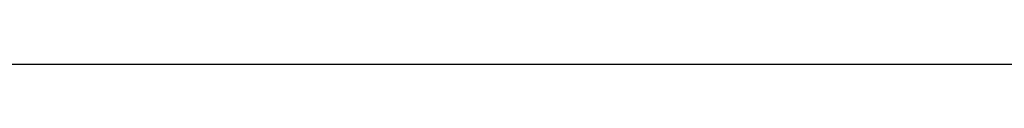
# Model space of a CAD drawing. Units: inches. Extents: x 459864 to 460310, y 324185 to 324787.
# Tile 100 of 112: x 460248.739 to 460250.864, y 324283.483 to 324283.483. Entities that reach past the tile are written whole.
import ezdxf

# ---------------------------------------------------------------- set-up
doc = ezdxf.new("R2010")
doc.units = ezdxf.units.IN
for name, color, linetype, lineweight in [('A-ANNO-DIMS', 2, 'Continuous', 18), ('L-HRDS', 9, 'Continuous', 18), ('L-SITE-PATT', 252, 'Continuous', 13)]:
    doc.layers.add(name, color=color, linetype=linetype, lineweight=lineweight)
doc.styles.get("Standard").update_dxf_attribs({"font": 'arial.ttf'})
doc.dimstyles.new('ISO-25', dxfattribs={"dimtxt": 6, "dimasz": 2.5, "dimexe": 1.25, "dimexo": 0.625, "dimtad": 1, "dimdec": 1, "dimlunit": 3, "dimtxsty": 'Standard', "dimcen": 2.5, "dimadec": 0, "dimazin": 0, "dimtfac": 1, "dimtdec": 1, "dimtmove": 0, "dimatfit": 3, "dimfxl": 1, "dimarcsym": 0})

# ---------------------------------------------------------------- blocks, each defined once
blk = doc.blocks.new('*D21')
at = {"layer": 'A-ANNO-DIMS', "color": 0, "lineweight": -2, "transparency": 16777216}
for p, q in [((460247.7399, 324715.4832), (460309.5804, 324715.4832)), ((460308.3304, 324712.9832), (460308.3304, 324285.9832)), ((460247.7399, 324283.4832), (460309.5804, 324283.4832))]:
    blk.add_line(p, q, dxfattribs=at)
at = {"layer": 'A-ANNO-DIMS', "color": 0, "transparency": 16777216}
for points in [[(460307.9137, 324712.9832), (460308.747, 324712.9832), (460308.3304, 324715.4832)], [(460307.9137, 324285.9832), (460308.747, 324285.9832), (460308.3304, 324283.4832)]]:
    blk.add_solid(points, dxfattribs=at)
at = {"layer": 'Defpoints', "color": 0, "transparency": 16777216}
for p in [(460247.1149, 324715.4832), (460247.1149, 324283.4832), (460308.3304, 324283.4832)]:
    blk.add_point(p, dxfattribs=at)
at = {"layer": 'A-ANNO-DIMS', "color": 0, "transparency": 16777216, "insert": (460304.6399, 324499.4832), "char_height": 6, "attachment_point": 5, "rotation": 90}
blk.add_mtext("36'", dxfattribs=at)

msp = doc.modelspace()

# ---------------------------------------------------------------- hatches: boundary and pattern name
at = {"layer": 'L-SITE-PATT'}
h = msp.add_hatch(dxfattribs=at)
h.set_pattern_fill('DOTS', color=256)
h.paths.add_polyline_path([(460269.8036, 324283.4832), (460247.1149, 324283.4832), (460121.9293, 324283.4832), (460121.9293, 324252.473), (460117.4293, 324252.473), (460110.1236, 324252.473), (460110.1236, 324243.2865), (460080.8295, 324243.2865), (460080.8295, 324252.473), (460061.1149, 324252.473), (460061.1149, 324251.8824), (460077.9089, 324251.8824), (460077.9089, 324199.4832), (460080.8295, 324199.4832), (460080.8295, 324207.5532), (460110.1236, 324207.5532), (460110.1236, 324199.4832), (460110.8133, 324199.4832), (460262.1149, 324199.4832), (460269.8036, 324199.4832)], flags=17)
edge = h.paths.add_edge_path(flags=0)
edge.add_ellipse((460222.5903, 324263.8132), major_axis=(-8.4853, 8.4853), ratio=1, start_angle=405, end_angle=495, ccw=False)
edge.add_line((460214.8209, 324254.6599), (460214.8316, 324254.6659))
edge.add_ellipse((460222.5903, 324263.8132), major_axis=(-8.4853, 8.4853), ratio=1, start_angle=405, end_angle=495, ccw=False)
edge.add_line((460210.7589, 324261.7806), (460210.7676, 324261.7868))
edge.add_ellipse((460222.5903, 324263.8132), major_axis=(-8.4853, 8.4853), ratio=1, start_angle=405, end_angle=495, ccw=False)
edge.add_ellipse((460222.5903, 324263.8132), major_axis=(-8.4853, 8.4853), ratio=1, start_angle=392.75402, end_angle=405, ccw=False)
edge.add_ellipse((460222.5903, 324263.8132), major_axis=(-8.4853, 8.4853), ratio=1, start_angle=380.93472, end_angle=392.75402, ccw=False)
edge.add_line((460211.3371, 324267.985), (460211.3404, 324267.985))
edge.add_ellipse((460222.5903, 324263.8132), major_axis=(-8.4853, 8.4853), ratio=1, start_angle=380.93472, end_angle=392.75402, ccw=False)
edge.add_ellipse((460222.5903, 324263.8132), major_axis=(-8.4853, 8.4853), ratio=1, start_angle=347.90152, end_angle=380.93472, ccw=False)
edge.add_ellipse((460222.5903, 324263.8132), major_axis=(-8.4853, 8.4853), ratio=1, start_angle=327.06192, end_angle=347.90152, ccw=False)
edge.add_ellipse((460222.5903, 324263.8132), major_axis=(-8.4853, 8.4853), ratio=1, start_angle=278.32464, end_angle=327.06192, ccw=False)
edge.add_line((460225.1583, 324275.536), (460225.1577, 324275.5346))
edge.add_ellipse((460222.5903, 324263.8132), major_axis=(-8.4853, 8.4853), ratio=1, start_angle=278.32464, end_angle=327.06192, ccw=False)
edge.add_ellipse((460222.5903, 324263.8132), major_axis=(-8.4853, 8.4853), ratio=1, start_angle=260.64357, end_angle=278.32464, ccw=False)
edge.add_ellipse((460222.5903, 324263.8132), major_axis=(-8.4853, 8.4853), ratio=1, start_angle=225, end_angle=260.64357, ccw=False)
edge.add_line((460234.5088, 324265.2428), (460234.5015, 324265.2394))
edge.add_ellipse((460222.5903, 324263.8132), major_axis=(-8.4853, 8.4853), ratio=1, start_angle=225, end_angle=260.64357, ccw=False)
edge.add_ellipse((460222.5903, 324263.8132), major_axis=(-8.4853, 8.4853), ratio=1, start_angle=495, end_angle=585, ccw=False)
edge.add_line((460234.4367, 324261.8612), (460234.4238, 324261.8578))
edge.add_ellipse((460222.5903, 324263.8132), major_axis=(-8.4853, 8.4853), ratio=1, start_angle=495, end_angle=585, ccw=False)
edge.add_line((460227.9501, 324253.0672), (460227.9464, 324253.0831))
edge.add_ellipse((460222.5903, 324263.8132), major_axis=(-8.4853, 8.4853), ratio=1, start_angle=495, end_angle=585, ccw=False)
edge.add_line((460226.223, 324252.3693), (460226.211, 324252.3796))
edge.add_ellipse((460222.5903, 324263.8132), major_axis=(-8.4853, 8.4853), ratio=1, start_angle=495, end_angle=585, ccw=False)
h.paths.add_polyline_path([(460219.6515, 324254.3467), (460218.4613, 324253.545), (460218.2754, 324254.7893), (460219.6424, 324256.5418), (460219.6246, 324260.8476), (460216.1101, 324257.333), (460214.35, 324256.9781), (460215.4164, 324259.3557), (460212.5239, 324258.4958), (460213.1373, 324259.9298), (460218.5072, 324263.8132), (460222.5903, 324263.8132), (460222.5903, 324267.8067), (460218.1755, 324272.2123), (460219.026, 324274.639), (460222.5903, 324272.8111), (460222.5903, 324275.4233), (460223.0571, 324274.8249), (460222.6752, 324273.4922), (460225.9117, 324267.1346), (460219.6246, 324260.8476)], flags=0)
edge = h.paths.add_edge_path(flags=0)
edge.add_ellipse((460194.5758, 324264.0465), major_axis=(-8.4853, 8.4853), ratio=1, start_angle=495, end_angle=585, ccw=False)
edge.add_line((460199.9356, 324253.3005), (460199.9319, 324253.3164))
edge.add_ellipse((460194.5758, 324264.0465), major_axis=(-8.4853, 8.4853), ratio=1, start_angle=495, end_angle=585, ccw=False)
edge.add_line((460198.2084, 324252.6025), (460198.1965, 324252.6128))
edge.add_ellipse((460194.5758, 324264.0465), major_axis=(-8.4853, 8.4853), ratio=1, start_angle=495, end_angle=585, ccw=False)
edge.add_ellipse((460194.5758, 324264.0465), major_axis=(-8.4853, 8.4853), ratio=1, start_angle=405, end_angle=495, ccw=False)
edge.add_line((460186.8063, 324254.8932), (460186.8171, 324254.8992))
edge.add_ellipse((460194.5758, 324264.0465), major_axis=(-8.4853, 8.4853), ratio=1, start_angle=405, end_angle=495, ccw=False)
edge.add_line((460182.7444, 324262.0138), (460182.753, 324262.0201))
edge.add_ellipse((460194.5758, 324264.0465), major_axis=(-8.4853, 8.4853), ratio=1, start_angle=405, end_angle=495, ccw=False)
edge.add_ellipse((460194.5758, 324264.0465), major_axis=(-8.4853, 8.4853), ratio=1, start_angle=392.75402, end_angle=405, ccw=False)
edge.add_ellipse((460194.5758, 324264.0465), major_axis=(-8.4853, 8.4853), ratio=1, start_angle=380.93472, end_angle=392.75402, ccw=False)
edge.add_line((460183.3225, 324268.2183), (460183.3259, 324268.2183))
edge.add_ellipse((460194.5758, 324264.0465), major_axis=(-8.4853, 8.4853), ratio=1, start_angle=380.93472, end_angle=392.75402, ccw=False)
edge.add_ellipse((460194.5758, 324264.0465), major_axis=(-8.4853, 8.4853), ratio=1, start_angle=347.90152, end_angle=380.93472, ccw=False)
edge.add_ellipse((460194.5758, 324264.0465), major_axis=(-8.4853, 8.4853), ratio=1, start_angle=327.06192, end_angle=347.90152, ccw=False)
edge.add_ellipse((460194.5758, 324264.0465), major_axis=(-8.4853, 8.4853), ratio=1, start_angle=278.32464, end_angle=327.06192, ccw=False)
edge.add_line((460197.1437, 324275.7693), (460197.1432, 324275.7679))
edge.add_ellipse((460194.5758, 324264.0465), major_axis=(-8.4853, 8.4853), ratio=1, start_angle=278.32464, end_angle=327.06192, ccw=False)
edge.add_ellipse((460194.5758, 324264.0465), major_axis=(-8.4853, 8.4853), ratio=1, start_angle=260.64357, end_angle=278.32464, ccw=False)
edge.add_ellipse((460194.5758, 324264.0465), major_axis=(-8.4853, 8.4853), ratio=1, start_angle=225, end_angle=260.64357, ccw=False)
edge.add_line((460206.4943, 324265.4761), (460206.4869, 324265.4727))
edge.add_ellipse((460194.5758, 324264.0465), major_axis=(-8.4853, 8.4853), ratio=1, start_angle=225, end_angle=260.64357, ccw=False)
edge.add_ellipse((460194.5758, 324264.0465), major_axis=(-8.4853, 8.4853), ratio=1, start_angle=495, end_angle=585, ccw=False)
edge.add_line((460206.4221, 324262.0945), (460206.4092, 324262.0911))
h.paths.add_polyline_path([(460191.6101, 324261.0808), (460191.6369, 324254.5799), (460190.4468, 324253.7783), (460190.2609, 324255.0226), (460191.6279, 324256.775), (460191.6101, 324261.0808), (460188.0956, 324257.5663), (460186.3354, 324257.2113), (460187.4018, 324259.5889), (460184.5094, 324258.7291), (460185.1228, 324260.1631), (460190.4927, 324264.0465), (460194.5758, 324264.0465), (460194.5758, 324268.04), (460190.161, 324272.4456), (460191.0114, 324274.8722), (460194.5758, 324273.0444), (460194.5758, 324275.6566), (460195.0426, 324275.0582), (460194.6607, 324273.7255), (460197.8971, 324267.3679)], flags=0)
edge = h.paths.add_edge_path(flags=0)
edge.add_ellipse((460252.912, 324263.5776), major_axis=(-8.4853, 8.4853), ratio=1, start_angle=405, end_angle=495, ccw=False)
edge.add_line((460241.0806, 324261.5449), (460241.0892, 324261.5512))
edge.add_ellipse((460252.912, 324263.5776), major_axis=(-8.4853, 8.4853), ratio=1, start_angle=405, end_angle=495, ccw=False)
edge.add_ellipse((460252.912, 324263.5776), major_axis=(-8.4853, 8.4853), ratio=1, start_angle=392.75402, end_angle=405, ccw=False)
edge.add_ellipse((460252.912, 324263.5776), major_axis=(-8.4853, 8.4853), ratio=1, start_angle=380.93472, end_angle=392.75402, ccw=False)
edge.add_line((460241.6587, 324267.7494), (460241.6621, 324267.7494))
edge.add_ellipse((460252.912, 324263.5776), major_axis=(-8.4853, 8.4853), ratio=1, start_angle=380.93472, end_angle=392.75402, ccw=False)
edge.add_ellipse((460252.912, 324263.5776), major_axis=(-8.4853, 8.4853), ratio=1, start_angle=347.90152, end_angle=380.93472, ccw=False)
edge.add_ellipse((460252.912, 324263.5776), major_axis=(-8.4853, 8.4853), ratio=1, start_angle=327.06192, end_angle=347.90152, ccw=False)
edge.add_ellipse((460252.912, 324263.5776), major_axis=(-8.4853, 8.4853), ratio=1, start_angle=278.32464, end_angle=327.06192, ccw=False)
edge.add_line((460255.4799, 324275.3004), (460255.4794, 324275.299))
edge.add_ellipse((460252.912, 324263.5776), major_axis=(-8.4853, 8.4853), ratio=1, start_angle=278.32464, end_angle=327.06192, ccw=False)
edge.add_ellipse((460252.912, 324263.5776), major_axis=(-8.4853, 8.4853), ratio=1, start_angle=260.64357, end_angle=278.32464, ccw=False)
edge.add_ellipse((460252.912, 324263.5776), major_axis=(-8.4853, 8.4853), ratio=1, start_angle=225, end_angle=260.64357, ccw=False)
edge.add_line((460264.8305, 324265.0072), (460264.8231, 324265.0038))
edge.add_ellipse((460252.912, 324263.5776), major_axis=(-8.4853, 8.4853), ratio=1, start_angle=225, end_angle=260.64357, ccw=False)
edge.add_ellipse((460252.912, 324263.5776), major_axis=(-8.4853, 8.4853), ratio=1, start_angle=495, end_angle=585, ccw=False)
edge.add_line((460264.7583, 324261.6256), (460264.7454, 324261.6222))
edge.add_ellipse((460252.912, 324263.5776), major_axis=(-8.4853, 8.4853), ratio=1, start_angle=495, end_angle=585, ccw=False)
edge.add_line((460258.2718, 324252.8316), (460258.2681, 324252.8475))
edge.add_ellipse((460252.912, 324263.5776), major_axis=(-8.4853, 8.4853), ratio=1, start_angle=495, end_angle=585, ccw=False)
edge.add_line((460256.5446, 324252.1337), (460256.5327, 324252.1439))
edge.add_ellipse((460252.912, 324263.5776), major_axis=(-8.4853, 8.4853), ratio=1, start_angle=495, end_angle=585, ccw=False)
edge.add_ellipse((460252.912, 324263.5776), major_axis=(-8.4853, 8.4853), ratio=1, start_angle=405, end_angle=495, ccw=False)
edge.add_line((460245.1425, 324254.4243), (460245.1533, 324254.4303))
h.paths.add_polyline_path([(460244.6716, 324256.7425), (460245.738, 324259.1201), (460242.8456, 324258.2602), (460243.459, 324259.6942), (460248.8289, 324263.5776), (460252.912, 324263.5776), (460252.912, 324267.5711), (460248.4972, 324271.9767), (460249.3476, 324274.4034), (460252.912, 324272.5755), (460252.912, 324275.1877), (460253.3788, 324274.5893), (460252.9969, 324273.2566), (460256.2333, 324266.899), (460249.9463, 324260.612), (460249.9731, 324254.111), (460248.783, 324253.3094), (460248.5971, 324254.5537), (460249.9641, 324256.3062), (460249.9463, 324260.612), (460246.4318, 324257.0974)], flags=0)
edge = h.paths.add_edge_path(flags=0)
edge.add_ellipse((460167.4387, 324262.8328), major_axis=(-8.4853, 8.4853), ratio=1, start_angle=495, end_angle=585, ccw=False)
edge.add_line((460172.7985, 324252.0868), (460172.7948, 324252.1027))
edge.add_ellipse((460167.4387, 324262.8328), major_axis=(-8.4853, 8.4853), ratio=1, start_angle=495, end_angle=585, ccw=False)
edge.add_line((460171.0714, 324251.3888), (460171.0594, 324251.3991))
edge.add_ellipse((460167.4387, 324262.8328), major_axis=(-8.4853, 8.4853), ratio=1, start_angle=495, end_angle=585, ccw=False)
edge.add_ellipse((460167.4387, 324262.8328), major_axis=(-8.4853, 8.4853), ratio=1, start_angle=405, end_angle=495, ccw=False)
edge.add_line((460159.6693, 324253.6795), (460159.68, 324253.6855))
edge.add_ellipse((460167.4387, 324262.8328), major_axis=(-8.4853, 8.4853), ratio=1, start_angle=405, end_angle=495, ccw=False)
edge.add_line((460155.6073, 324260.8001), (460155.616, 324260.8064))
edge.add_ellipse((460167.4387, 324262.8328), major_axis=(-8.4853, 8.4853), ratio=1, start_angle=405, end_angle=495, ccw=False)
edge.add_ellipse((460167.4387, 324262.8328), major_axis=(-8.4853, 8.4853), ratio=1, start_angle=392.75402, end_angle=405, ccw=False)
edge.add_ellipse((460167.4387, 324262.8328), major_axis=(-8.4853, 8.4853), ratio=1, start_angle=380.93472, end_angle=392.75402, ccw=False)
edge.add_line((460156.1855, 324267.0046), (460156.1888, 324267.0046))
edge.add_ellipse((460167.4387, 324262.8328), major_axis=(-8.4853, 8.4853), ratio=1, start_angle=380.93472, end_angle=392.75402, ccw=False)
edge.add_ellipse((460167.4387, 324262.8328), major_axis=(-8.4853, 8.4853), ratio=1, start_angle=347.90152, end_angle=380.93472, ccw=False)
edge.add_ellipse((460167.4387, 324262.8328), major_axis=(-8.4853, 8.4853), ratio=1, start_angle=327.06192, end_angle=347.90152, ccw=False)
edge.add_ellipse((460167.4387, 324262.8328), major_axis=(-8.4853, 8.4853), ratio=1, start_angle=278.32464, end_angle=327.06192, ccw=False)
edge.add_line((460170.0067, 324274.5556), (460170.0061, 324274.5542))
edge.add_ellipse((460167.4387, 324262.8328), major_axis=(-8.4853, 8.4853), ratio=1, start_angle=278.32464, end_angle=327.06192, ccw=False)
edge.add_ellipse((460167.4387, 324262.8328), major_axis=(-8.4853, 8.4853), ratio=1, start_angle=260.64357, end_angle=278.32464, ccw=False)
edge.add_ellipse((460167.4387, 324262.8328), major_axis=(-8.4853, 8.4853), ratio=1, start_angle=225, end_angle=260.64357, ccw=False)
edge.add_line((460179.3572, 324264.2624), (460179.3499, 324264.259))
edge.add_ellipse((460167.4387, 324262.8328), major_axis=(-8.4853, 8.4853), ratio=1, start_angle=225, end_angle=260.64357, ccw=False)
edge.add_ellipse((460167.4387, 324262.8328), major_axis=(-8.4853, 8.4853), ratio=1, start_angle=495, end_angle=585, ccw=False)
edge.add_line((460179.2851, 324260.8808), (460179.2722, 324260.8774))
h.paths.add_polyline_path([(460164.473, 324259.8671), (460164.4998, 324253.3662), (460163.3097, 324252.5645), (460163.1238, 324253.8089), (460164.4908, 324255.5613), (460164.473, 324259.8671), (460160.9585, 324256.3526), (460159.1984, 324255.9976), (460160.2648, 324258.3752), (460157.3723, 324257.5154), (460157.9857, 324258.9494), (460163.3556, 324262.8328), (460167.4387, 324262.8328), (460167.4387, 324266.8263), (460163.0239, 324271.2319), (460163.8744, 324273.6585), (460167.4387, 324271.8307), (460167.4387, 324274.4429), (460167.9055, 324273.8445), (460167.5236, 324272.5118), (460170.7601, 324266.1542)], flags=0)
edge = h.paths.add_edge_path(flags=0)
edge.add_ellipse((460140.7581, 324262.3696), major_axis=(-8.4853, 8.4853), ratio=1, start_angle=495, end_angle=585, ccw=False)
edge.add_line((460146.1179, 324251.6235), (460146.1142, 324251.6395))
edge.add_ellipse((460140.7581, 324262.3696), major_axis=(-8.4853, 8.4853), ratio=1, start_angle=495, end_angle=585, ccw=False)
edge.add_line((460144.3908, 324250.9256), (460144.3788, 324250.9359))
edge.add_ellipse((460140.7581, 324262.3696), major_axis=(-8.4853, 8.4853), ratio=1, start_angle=495, end_angle=585, ccw=False)
edge.add_ellipse((460140.7581, 324262.3696), major_axis=(-8.4853, 8.4853), ratio=1, start_angle=405, end_angle=495, ccw=False)
edge.add_line((460132.9887, 324253.2162), (460132.9994, 324253.2223))
edge.add_ellipse((460140.7581, 324262.3696), major_axis=(-8.4853, 8.4853), ratio=1, start_angle=405, end_angle=495, ccw=False)
edge.add_line((460128.9267, 324260.3369), (460128.9354, 324260.3432))
edge.add_ellipse((460140.7581, 324262.3696), major_axis=(-8.4853, 8.4853), ratio=1, start_angle=405, end_angle=495, ccw=False)
edge.add_ellipse((460140.7581, 324262.3696), major_axis=(-8.4853, 8.4853), ratio=1, start_angle=392.75402, end_angle=405, ccw=False)
edge.add_ellipse((460140.7581, 324262.3696), major_axis=(-8.4853, 8.4853), ratio=1, start_angle=380.93472, end_angle=392.75402, ccw=False)
edge.add_line((460129.5049, 324266.5414), (460129.5082, 324266.5414))
edge.add_ellipse((460140.7581, 324262.3696), major_axis=(-8.4853, 8.4853), ratio=1, start_angle=380.93472, end_angle=392.75402, ccw=False)
edge.add_ellipse((460140.7581, 324262.3696), major_axis=(-8.4853, 8.4853), ratio=1, start_angle=347.90152, end_angle=380.93472, ccw=False)
edge.add_ellipse((460140.7581, 324262.3696), major_axis=(-8.4853, 8.4853), ratio=1, start_angle=327.06192, end_angle=347.90152, ccw=False)
edge.add_ellipse((460140.7581, 324262.3696), major_axis=(-8.4853, 8.4853), ratio=1, start_angle=278.32464, end_angle=327.06192, ccw=False)
edge.add_line((460143.3261, 324274.0923), (460143.3255, 324274.091))
edge.add_ellipse((460140.7581, 324262.3696), major_axis=(-8.4853, 8.4853), ratio=1, start_angle=278.32464, end_angle=327.06192, ccw=False)
edge.add_ellipse((460140.7581, 324262.3696), major_axis=(-8.4853, 8.4853), ratio=1, start_angle=260.64357, end_angle=278.32464, ccw=False)
edge.add_ellipse((460140.7581, 324262.3696), major_axis=(-8.4853, 8.4853), ratio=1, start_angle=225, end_angle=260.64357, ccw=False)
edge.add_line((460152.6766, 324263.7992), (460152.6692, 324263.7958))
edge.add_ellipse((460140.7581, 324262.3696), major_axis=(-8.4853, 8.4853), ratio=1, start_angle=225, end_angle=260.64357, ccw=False)
edge.add_ellipse((460140.7581, 324262.3696), major_axis=(-8.4853, 8.4853), ratio=1, start_angle=495, end_angle=585, ccw=False)
edge.add_line((460152.6045, 324260.4176), (460152.5916, 324260.4142))
h.paths.add_polyline_path([(460137.7924, 324259.4039), (460137.8192, 324252.903), (460136.6291, 324252.1013), (460136.4432, 324253.3457), (460137.8102, 324255.0981), (460137.7924, 324259.4039), (460134.2779, 324255.8894), (460132.5178, 324255.5344), (460133.5842, 324257.912), (460130.6917, 324257.0522), (460131.3051, 324258.4862), (460136.675, 324262.3696), (460140.7581, 324262.3696), (460140.7581, 324266.3631), (460136.3433, 324270.7687), (460137.1938, 324273.1953), (460140.7581, 324271.3675), (460140.7581, 324273.9797), (460141.2249, 324273.3813), (460140.843, 324272.0486), (460144.0795, 324265.691)], flags=0)
h.paths.add_polyline_path([(460110.1236, 324227.4139), (460080.8295, 324227.4139), (460080.8295, 324235.4839), (460110.1236, 324235.4839)], flags=16)
h.paths.add_polyline_path([(460110.1236, 324220.7966), (460110.1236, 324212.7267), (460080.8295, 324212.7267), (460080.8295, 324220.7966)], flags=16)
h.paths.add_polyline_path([(460269.8036, 324283.4832), (460247.1149, 324283.4832), (460121.9293, 324283.4832), (460121.9293, 324252.473), (460117.4293, 324252.473), (460110.1236, 324252.473), (460110.1236, 324243.2865), (460080.8295, 324243.2865), (460080.8295, 324252.473), (460061.1149, 324252.473), (460061.1149, 324251.8824), (460077.9089, 324251.8824), (460077.9089, 324199.4832), (460080.8295, 324199.4832), (460080.8295, 324207.5532), (460110.1236, 324207.5532), (460110.1236, 324199.4832), (460262.1149, 324199.4832), (460269.8036, 324199.4832)], flags=17)
h.paths.add_polyline_path([(460219.6515, 324254.3467), (460218.4613, 324253.545), (460218.2754, 324254.7893), (460219.6424, 324256.5418), (460219.6246, 324260.8476), (460216.1101, 324257.333), (460214.35, 324256.9781), (460215.4164, 324259.3557), (460212.5239, 324258.4958), (460213.1373, 324259.9298), (460218.5072, 324263.8132), (460222.5903, 324263.8132), (460220.1805, 324266.223), (460215.461, 324265.3076), (460211.8345, 324266.1366), (460216.2466, 324267.985), (460218.4185, 324267.985), (460222.5903, 324263.8132), (460222.5903, 324267.8067), (460218.1755, 324272.2123), (460219.026, 324274.639), (460222.5903, 324272.8111), (460222.5903, 324275.4233), (460223.0571, 324274.8249), (460222.6752, 324273.4922), (460225.9117, 324267.1346), (460222.5903, 324263.8132), (460231.3829, 324263.8132), (460228.4847, 324262.4878), (460224.4252, 324261.9783), (460228.6799, 324257.7236), (460228.9658, 324254.791), (460227.1418, 324256.5366), (460227.5421, 324254.8186), (460227.3333, 324253.6145), (460222.5903, 324259.9846), (460222.5903, 324255.4967), (460221.3774, 324256.5408), (460220.5758, 324261.7987), (460219.6246, 324260.8476)], flags=0)
h.paths.add_polyline_path([(460199.1272, 324256.7699), (460199.5275, 324255.0518), (460199.3188, 324253.8477), (460194.5758, 324260.2179), (460194.5758, 324255.7299), (460193.3629, 324256.7741), (460192.5613, 324262.032), (460191.6101, 324261.0808), (460191.6369, 324254.5799), (460190.4468, 324253.7783), (460190.2609, 324255.0226), (460191.6279, 324256.775), (460191.6101, 324261.0808), (460188.0956, 324257.5663), (460186.3354, 324257.2113), (460187.4018, 324259.5889), (460184.5094, 324258.7291), (460185.1228, 324260.1631), (460190.4927, 324264.0465), (460194.5758, 324264.0465), (460192.1659, 324266.4563), (460187.4464, 324265.5409), (460183.82, 324266.3698), (460188.2321, 324268.2183), (460190.404, 324268.2183), (460194.5758, 324264.0465), (460194.5758, 324268.04), (460190.161, 324272.4456), (460191.0114, 324274.8722), (460194.5758, 324273.0444), (460194.5758, 324275.6566), (460195.0426, 324275.0582), (460194.6607, 324273.7255), (460197.8971, 324267.3679), (460194.5758, 324264.0465), (460203.3683, 324264.0465), (460200.4702, 324262.7211), (460196.4107, 324262.2116), (460200.6654, 324257.9569), (460200.9513, 324255.0243)], flags=0)
h.paths.add_polyline_path([(460244.6716, 324256.7425), (460245.738, 324259.1201), (460242.8456, 324258.2602), (460243.459, 324259.6942), (460248.8289, 324263.5776), (460252.912, 324263.5776), (460250.5022, 324265.9874), (460245.7826, 324265.072), (460242.1562, 324265.9009), (460246.5683, 324267.7494), (460248.7402, 324267.7494), (460252.912, 324263.5776), (460252.912, 324267.5711), (460248.4972, 324271.9767), (460249.3476, 324274.4034), (460252.912, 324272.5755), (460252.912, 324275.1877), (460253.3788, 324274.5893), (460252.9969, 324273.2566), (460256.2333, 324266.899), (460252.912, 324263.5776), (460261.7045, 324263.5776), (460258.8064, 324262.2522), (460254.7469, 324261.7427), (460259.0016, 324257.488), (460259.2875, 324254.5554), (460257.4634, 324256.301), (460257.8637, 324254.583), (460257.655, 324253.3789), (460252.912, 324259.749), (460252.912, 324255.2611), (460251.6991, 324256.3052), (460250.8975, 324261.5631), (460249.9463, 324260.612), (460249.9731, 324254.111), (460248.783, 324253.3094), (460248.5971, 324254.5537), (460249.9641, 324256.3062), (460249.9463, 324260.612), (460246.4318, 324257.0974)], flags=0)
h.paths.add_polyline_path([(460173.5283, 324256.7432), (460173.8142, 324253.8106), (460171.9902, 324255.5562), (460172.3905, 324253.8381), (460172.1817, 324252.634), (460167.4387, 324259.0042), (460167.4387, 324254.5162), (460166.2258, 324255.5604), (460165.4242, 324260.8183), (460164.473, 324259.8671), (460164.4998, 324253.3662), (460163.3097, 324252.5645), (460163.1238, 324253.8089), (460164.4908, 324255.5613), (460164.473, 324259.8671), (460160.9585, 324256.3526), (460159.1984, 324255.9976), (460160.2648, 324258.3752), (460157.3723, 324257.5154), (460157.9857, 324258.9494), (460163.3556, 324262.8328), (460167.4387, 324262.8328), (460165.0289, 324265.2426), (460160.3094, 324264.3272), (460156.6829, 324265.1561), (460161.095, 324267.0046), (460163.2669, 324267.0046), (460167.4387, 324262.8328), (460167.4387, 324266.8263), (460163.0239, 324271.2319), (460163.8744, 324273.6585), (460167.4387, 324271.8307), (460167.4387, 324274.4429), (460167.9055, 324273.8445), (460167.5236, 324272.5118), (460170.7601, 324266.1542), (460167.4387, 324262.8328), (460176.2313, 324262.8328), (460173.3331, 324261.5074), (460169.2736, 324260.9979)], flags=0)
h.paths.add_polyline_path([(460146.8477, 324256.28), (460147.1336, 324253.3474), (460145.3096, 324255.093), (460145.7099, 324253.3749), (460145.5011, 324252.1708), (460140.7581, 324258.541), (460140.7581, 324254.053), (460139.5452, 324255.0972), (460138.7436, 324260.3551), (460137.7924, 324259.4039), (460137.8192, 324252.903), (460136.6291, 324252.1013), (460136.4432, 324253.3457), (460137.8102, 324255.0981), (460137.7924, 324259.4039), (460134.2779, 324255.8894), (460132.5178, 324255.5344), (460133.5842, 324257.912), (460130.6917, 324257.0522), (460131.3051, 324258.4862), (460136.675, 324262.3696), (460140.7581, 324262.3696), (460138.3483, 324264.7794), (460133.6288, 324263.864), (460130.0023, 324264.6929), (460134.4144, 324266.5414), (460136.5863, 324266.5414), (460140.7581, 324262.3696), (460140.7581, 324266.3631), (460136.3433, 324270.7687), (460137.1938, 324273.1953), (460140.7581, 324271.3675), (460140.7581, 324273.9797), (460141.2249, 324273.3813), (460140.843, 324272.0486), (460144.0795, 324265.691), (460140.7581, 324262.3696), (460149.5507, 324262.3696), (460146.6525, 324261.0442), (460142.593, 324260.5347)], flags=0)
edge = h.paths.add_edge_path()
edge.add_line((460269.8036, 324272.5491), (460260.8815, 324272.5491))
edge.add_ellipse((460252.912, 324263.5776), major_axis=(-8.4853, 8.4853), ratio=1, start_angle=260.64357, end_angle=273.38462, ccw=False)
edge.add_line((460262.2826, 324271.0921), (460262.2606, 324271.0911))
edge.add_ellipse((460252.912, 324263.5776), major_axis=(-8.4853, 8.4853), ratio=1, start_angle=260.64357, end_angle=273.38462, ccw=False)
edge.add_ellipse((460252.912, 324263.5776), major_axis=(-8.4853, 8.4853), ratio=1, start_angle=225, end_angle=260.64357, ccw=False)
edge.add_line((460263.6086, 324269.0633), (460263.5717, 324269.0583))
edge.add_ellipse((460252.912, 324263.5776), major_axis=(-8.4853, 8.4853), ratio=1, start_angle=225, end_angle=260.64357, ccw=False)
edge.add_line((460264.6155, 324266.3055), (460264.5854, 324266.3052))
edge.add_ellipse((460252.912, 324263.5776), major_axis=(-8.4853, 8.4853), ratio=1, start_angle=225, end_angle=260.64357, ccw=False)
edge.add_line((460264.8305, 324265.0072), (460264.8231, 324265.0038))
edge.add_ellipse((460252.912, 324263.5776), major_axis=(-8.4853, 8.4853), ratio=1, start_angle=225, end_angle=260.64357, ccw=False)
edge.add_ellipse((460252.912, 324263.5776), major_axis=(-8.4853, 8.4853), ratio=1, start_angle=495, end_angle=585, ccw=False)
edge.add_line((460264.7583, 324261.6256), (460264.7454, 324261.6222))
edge.add_ellipse((460252.912, 324263.5776), major_axis=(-8.4853, 8.4853), ratio=1, start_angle=495, end_angle=585, ccw=False)
edge.add_line((460263.4422, 324257.739), (460263.3893, 324257.7792))
edge.add_ellipse((460252.912, 324263.5776), major_axis=(-8.4853, 8.4853), ratio=1, start_angle=495, end_angle=585, ccw=False)
edge.add_line((460258.1281, 324252.7435), (460258.1019, 324252.7787))
edge.add_ellipse((460252.912, 324263.5776), major_axis=(-8.4853, 8.4853), ratio=1, start_angle=495, end_angle=585, ccw=False)
edge.add_line((460256.5446, 324252.1337), (460256.5327, 324252.1439))
edge.add_ellipse((460252.912, 324263.5776), major_axis=(-8.4853, 8.4853), ratio=1, start_angle=495, end_angle=585, ccw=False)
edge.add_ellipse((460252.912, 324263.5776), major_axis=(-8.4853, 8.4853), ratio=1, start_angle=405, end_angle=495, ccw=False)
edge.add_line((460250.594, 324251.7804), (460250.6047, 324251.8198))
edge.add_ellipse((460252.912, 324263.5776), major_axis=(-8.4853, 8.4853), ratio=1, start_angle=405, end_angle=495, ccw=False)
edge.add_line((460245.1425, 324254.4243), (460245.1533, 324254.4303))
edge.add_ellipse((460252.912, 324263.5776), major_axis=(-8.4853, 8.4853), ratio=1, start_angle=405, end_angle=495, ccw=False)
edge.add_line((460243.5246, 324256.059), (460243.5603, 324256.0914))
edge.add_ellipse((460252.912, 324263.5776), major_axis=(-8.4853, 8.4853), ratio=1, start_angle=405, end_angle=495, ccw=False)
edge.add_line((460241.4401, 324259.8927), (460241.5224, 324259.8959))
edge.add_ellipse((460252.912, 324263.5776), major_axis=(-8.4853, 8.4853), ratio=1, start_angle=405, end_angle=495, ccw=False)
edge.add_line((460241.0806, 324261.5449), (460241.0892, 324261.5512))
edge.add_ellipse((460252.912, 324263.5776), major_axis=(-8.4853, 8.4853), ratio=1, start_angle=405, end_angle=495, ccw=False)
edge.add_ellipse((460252.912, 324263.5776), major_axis=(-8.4853, 8.4853), ratio=1, start_angle=392.75402, end_angle=405, ccw=False)
edge.add_line((460241.0503, 324265.4376), (460241.0626, 324265.4428))
edge.add_ellipse((460252.912, 324263.5776), major_axis=(-8.4853, 8.4853), ratio=1, start_angle=392.75402, end_angle=405, ccw=False)
edge.add_ellipse((460252.912, 324263.5776), major_axis=(-8.4853, 8.4853), ratio=1, start_angle=380.93472, end_angle=392.75402, ccw=False)
edge.add_line((460241.4519, 324267.1764), (460241.469, 324267.171))
edge.add_ellipse((460252.912, 324263.5776), major_axis=(-8.4853, 8.4853), ratio=1, start_angle=380.93472, end_angle=392.75402, ccw=False)
edge.add_line((460241.6587, 324267.7494), (460241.6621, 324267.7494))
edge.add_ellipse((460252.912, 324263.5776), major_axis=(-8.4853, 8.4853), ratio=1, start_angle=380.93472, end_angle=392.75402, ccw=False)
edge.add_ellipse((460252.912, 324263.5776), major_axis=(-8.4853, 8.4853), ratio=1, start_angle=356.61538, end_angle=380.93472, ccw=False)
edge.add_line((460244.8803, 324272.4877), (460244.7127, 324272.5491))
edge.add_line((460244.7127, 324272.5491), (460230.8174, 324272.5491))
edge.add_ellipse((460222.5903, 324263.8132), major_axis=(-8.4853, 8.4853), ratio=1, start_angle=260.64357, end_angle=271.71777, ccw=False)
edge.add_ellipse((460222.5903, 324263.8132), major_axis=(-8.4853, 8.4853), ratio=1, start_angle=225, end_angle=260.64357, ccw=False)
edge.add_line((460233.2869, 324269.2989), (460233.25, 324269.2939))
edge.add_ellipse((460222.5903, 324263.8132), major_axis=(-8.4853, 8.4853), ratio=1, start_angle=225, end_angle=260.64357, ccw=False)
edge.add_line((460234.2938, 324266.5412), (460234.2637, 324266.5408))
edge.add_ellipse((460222.5903, 324263.8132), major_axis=(-8.4853, 8.4853), ratio=1, start_angle=225, end_angle=260.64357, ccw=False)
edge.add_line((460234.5088, 324265.2428), (460234.5015, 324265.2394))
edge.add_ellipse((460222.5903, 324263.8132), major_axis=(-8.4853, 8.4853), ratio=1, start_angle=225, end_angle=260.64357, ccw=False)
edge.add_ellipse((460222.5903, 324263.8132), major_axis=(-8.4853, 8.4853), ratio=1, start_angle=495, end_angle=585, ccw=False)
edge.add_line((460234.4367, 324261.8612), (460234.4238, 324261.8578))
edge.add_ellipse((460222.5903, 324263.8132), major_axis=(-8.4853, 8.4853), ratio=1, start_angle=495, end_angle=585, ccw=False)
edge.add_line((460233.1205, 324257.9746), (460233.0676, 324258.0149))
edge.add_ellipse((460222.5903, 324263.8132), major_axis=(-8.4853, 8.4853), ratio=1, start_angle=495, end_angle=585, ccw=False)
edge.add_line((460227.8064, 324252.9791), (460227.7802, 324253.0143))
edge.add_ellipse((460222.5903, 324263.8132), major_axis=(-8.4853, 8.4853), ratio=1, start_angle=495, end_angle=585, ccw=False)
edge.add_line((460226.223, 324252.3693), (460226.211, 324252.3796))
edge.add_ellipse((460222.5903, 324263.8132), major_axis=(-8.4853, 8.4853), ratio=1, start_angle=495, end_angle=585, ccw=False)
edge.add_ellipse((460222.5903, 324263.8132), major_axis=(-8.4853, 8.4853), ratio=1, start_angle=405, end_angle=495, ccw=False)
edge.add_line((460220.2723, 324252.016), (460220.283, 324252.0554))
edge.add_ellipse((460222.5903, 324263.8132), major_axis=(-8.4853, 8.4853), ratio=1, start_angle=405, end_angle=495, ccw=False)
edge.add_line((460214.8209, 324254.6599), (460214.8316, 324254.6659))
edge.add_ellipse((460222.5903, 324263.8132), major_axis=(-8.4853, 8.4853), ratio=1, start_angle=405, end_angle=495, ccw=False)
edge.add_line((460213.2029, 324256.2946), (460213.2387, 324256.327))
edge.add_ellipse((460222.5903, 324263.8132), major_axis=(-8.4853, 8.4853), ratio=1, start_angle=405, end_angle=495, ccw=False)
edge.add_line((460211.1184, 324260.1283), (460211.2008, 324260.1315))
edge.add_ellipse((460222.5903, 324263.8132), major_axis=(-8.4853, 8.4853), ratio=1, start_angle=405, end_angle=495, ccw=False)
edge.add_line((460210.7589, 324261.7806), (460210.7676, 324261.7868))
edge.add_ellipse((460222.5903, 324263.8132), major_axis=(-8.4853, 8.4853), ratio=1, start_angle=405, end_angle=495, ccw=False)
edge.add_ellipse((460222.5903, 324263.8132), major_axis=(-8.4853, 8.4853), ratio=1, start_angle=392.75402, end_angle=405, ccw=False)
edge.add_line((460210.7286, 324265.6732), (460210.7409, 324265.6784))
edge.add_ellipse((460222.5903, 324263.8132), major_axis=(-8.4853, 8.4853), ratio=1, start_angle=392.75402, end_angle=405, ccw=False)
edge.add_ellipse((460222.5903, 324263.8132), major_axis=(-8.4853, 8.4853), ratio=1, start_angle=380.93472, end_angle=392.75402, ccw=False)
edge.add_line((460211.1302, 324267.412), (460211.1474, 324267.4066))
edge.add_ellipse((460222.5903, 324263.8132), major_axis=(-8.4853, 8.4853), ratio=1, start_angle=380.93472, end_angle=392.75402, ccw=False)
edge.add_line((460211.3371, 324267.985), (460211.3404, 324267.985))
edge.add_ellipse((460222.5903, 324263.8132), major_axis=(-8.4853, 8.4853), ratio=1, start_angle=380.93472, end_angle=392.75402, ccw=False)
edge.add_ellipse((460222.5903, 324263.8132), major_axis=(-8.4853, 8.4853), ratio=1, start_angle=358.28223, end_angle=380.93472, ccw=False)
edge.add_line((460213.7045, 324271.9018), (460213.709, 324271.869))
edge.add_ellipse((460222.5903, 324263.8132), major_axis=(-8.4853, 8.4853), ratio=1, start_angle=358.28223, end_angle=380.93472, ccw=False)
edge.add_line((460214.3632, 324272.5491), (460203.0783, 324272.5491))
edge.add_line((460203.0783, 324272.5491), (460203.0603, 324272.5311))
edge.add_ellipse((460194.5758, 324264.0465), major_axis=(-8.4853, 8.4853), ratio=1, start_angle=260.64357, end_angle=270.11679, ccw=False)
edge.add_line((460203.9566, 324271.5615), (460203.9209, 324271.5598))
edge.add_ellipse((460194.5758, 324264.0465), major_axis=(-8.4853, 8.4853), ratio=1, start_angle=260.64357, end_angle=270.11679, ccw=False)
edge.add_ellipse((460194.5758, 324264.0465), major_axis=(-8.4853, 8.4853), ratio=1, start_angle=225, end_angle=260.64357, ccw=False)
edge.add_line((460205.2724, 324269.5322), (460205.2354, 324269.5272))
edge.add_ellipse((460194.5758, 324264.0465), major_axis=(-8.4853, 8.4853), ratio=1, start_angle=225, end_angle=260.64357, ccw=False)
edge.add_line((460206.2793, 324266.7744), (460206.2492, 324266.7741))
edge.add_ellipse((460194.5758, 324264.0465), major_axis=(-8.4853, 8.4853), ratio=1, start_angle=225, end_angle=260.64357, ccw=False)
edge.add_line((460206.4943, 324265.4761), (460206.4869, 324265.4727))
edge.add_ellipse((460194.5758, 324264.0465), major_axis=(-8.4853, 8.4853), ratio=1, start_angle=225, end_angle=260.64357, ccw=False)
edge.add_ellipse((460194.5758, 324264.0465), major_axis=(-8.4853, 8.4853), ratio=1, start_angle=495, end_angle=585, ccw=False)
edge.add_line((460206.4221, 324262.0945), (460206.4092, 324262.0911))
edge.add_ellipse((460194.5758, 324264.0465), major_axis=(-8.4853, 8.4853), ratio=1, start_angle=495, end_angle=585, ccw=False)
edge.add_line((460205.106, 324258.2079), (460205.0531, 324258.2481))
edge.add_ellipse((460194.5758, 324264.0465), major_axis=(-8.4853, 8.4853), ratio=1, start_angle=495, end_angle=585, ccw=False)
edge.add_line((460199.7919, 324253.2124), (460199.7657, 324253.2476))
edge.add_ellipse((460194.5758, 324264.0465), major_axis=(-8.4853, 8.4853), ratio=1, start_angle=495, end_angle=585, ccw=False)
edge.add_line((460198.2084, 324252.6025), (460198.1965, 324252.6128))
edge.add_ellipse((460194.5758, 324264.0465), major_axis=(-8.4853, 8.4853), ratio=1, start_angle=495, end_angle=585, ccw=False)
edge.add_ellipse((460194.5758, 324264.0465), major_axis=(-8.4853, 8.4853), ratio=1, start_angle=405, end_angle=495, ccw=False)
edge.add_line((460192.2578, 324252.2493), (460192.2684, 324252.2887))
edge.add_ellipse((460194.5758, 324264.0465), major_axis=(-8.4853, 8.4853), ratio=1, start_angle=405, end_angle=495, ccw=False)
edge.add_line((460186.8063, 324254.8932), (460186.8171, 324254.8992))
edge.add_ellipse((460194.5758, 324264.0465), major_axis=(-8.4853, 8.4853), ratio=1, start_angle=405, end_angle=495, ccw=False)
edge.add_line((460185.1884, 324256.5279), (460185.2241, 324256.5602))
edge.add_ellipse((460194.5758, 324264.0465), major_axis=(-8.4853, 8.4853), ratio=1, start_angle=405, end_angle=495, ccw=False)
edge.add_line((460183.1039, 324260.3616), (460183.1862, 324260.3648))
edge.add_ellipse((460194.5758, 324264.0465), major_axis=(-8.4853, 8.4853), ratio=1, start_angle=405, end_angle=495, ccw=False)
edge.add_line((460182.7444, 324262.0138), (460182.753, 324262.0201))
edge.add_ellipse((460194.5758, 324264.0465), major_axis=(-8.4853, 8.4853), ratio=1, start_angle=405, end_angle=495, ccw=False)
edge.add_ellipse((460194.5758, 324264.0465), major_axis=(-8.4853, 8.4853), ratio=1, start_angle=392.75402, end_angle=405, ccw=False)
edge.add_line((460182.7141, 324265.9065), (460182.7264, 324265.9116))
edge.add_ellipse((460194.5758, 324264.0465), major_axis=(-8.4853, 8.4853), ratio=1, start_angle=392.75402, end_angle=405, ccw=False)
edge.add_ellipse((460194.5758, 324264.0465), major_axis=(-8.4853, 8.4853), ratio=1, start_angle=380.93472, end_angle=392.75402, ccw=False)
edge.add_line((460183.1157, 324267.6453), (460183.1328, 324267.6399))
edge.add_ellipse((460194.5758, 324264.0465), major_axis=(-8.4853, 8.4853), ratio=1, start_angle=380.93472, end_angle=392.75402, ccw=False)
edge.add_line((460183.3225, 324268.2183), (460183.3259, 324268.2183))
edge.add_ellipse((460194.5758, 324264.0465), major_axis=(-8.4853, 8.4853), ratio=1, start_angle=380.93472, end_angle=392.75402, ccw=False)
edge.add_ellipse((460194.5758, 324264.0465), major_axis=(-8.4853, 8.4853), ratio=1, start_angle=359.88321, end_angle=380.93472, ccw=False)
edge.add_line((460184.4914, 324270.6108), (460184.5531, 324270.6108))
edge.add_ellipse((460194.5758, 324264.0465), major_axis=(-8.4853, 8.4853), ratio=1, start_angle=359.88321, end_angle=380.93472, ccw=False)
edge.add_line((460185.3458, 324271.7602), (460185.3786, 324271.728))
edge.add_ellipse((460194.5758, 324264.0465), major_axis=(-8.4853, 8.4853), ratio=1, start_angle=359.88321, end_angle=380.93472, ccw=False)
edge.add_line((460185.6967, 324272.0862), (460185.633, 324272.5491))
edge.add_line((460185.633, 324272.5491), (460174.6834, 324272.5491))
edge.add_line((460174.6834, 324272.5491), (460174.6061, 324272.4572))
edge.add_ellipse((460167.4387, 324262.8328), major_axis=(-8.4853, 8.4853), ratio=1, start_angle=260.64357, end_angle=278.32464, ccw=False)
edge.add_ellipse((460167.4387, 324262.8328), major_axis=(-8.4853, 8.4853), ratio=1, start_angle=225, end_angle=260.64357, ccw=False)
edge.add_line((460178.1353, 324268.3185), (460178.0984, 324268.3135))
edge.add_ellipse((460167.4387, 324262.8328), major_axis=(-8.4853, 8.4853), ratio=1, start_angle=225, end_angle=260.64357, ccw=False)
edge.add_line((460179.1422, 324265.5607), (460179.1121, 324265.5604))
edge.add_ellipse((460167.4387, 324262.8328), major_axis=(-8.4853, 8.4853), ratio=1, start_angle=225, end_angle=260.64357, ccw=False)
edge.add_line((460179.3572, 324264.2624), (460179.3499, 324264.259))
edge.add_ellipse((460167.4387, 324262.8328), major_axis=(-8.4853, 8.4853), ratio=1, start_angle=225, end_angle=260.64357, ccw=False)
edge.add_ellipse((460167.4387, 324262.8328), major_axis=(-8.4853, 8.4853), ratio=1, start_angle=495, end_angle=585, ccw=False)
edge.add_line((460179.2851, 324260.8808), (460179.2722, 324260.8774))
edge.add_ellipse((460167.4387, 324262.8328), major_axis=(-8.4853, 8.4853), ratio=1, start_angle=495, end_angle=585, ccw=False)
edge.add_line((460177.9689, 324256.9942), (460177.916, 324257.0344))
edge.add_ellipse((460167.4387, 324262.8328), major_axis=(-8.4853, 8.4853), ratio=1, start_angle=495, end_angle=585, ccw=False)
edge.add_line((460172.6548, 324251.9987), (460172.6286, 324252.0339))
edge.add_ellipse((460167.4387, 324262.8328), major_axis=(-8.4853, 8.4853), ratio=1, start_angle=495, end_angle=585, ccw=False)
edge.add_line((460171.0714, 324251.3888), (460171.0594, 324251.3991))
edge.add_ellipse((460167.4387, 324262.8328), major_axis=(-8.4853, 8.4853), ratio=1, start_angle=495, end_angle=585, ccw=False)
edge.add_ellipse((460167.4387, 324262.8328), major_axis=(-8.4853, 8.4853), ratio=1, start_angle=405, end_angle=495, ccw=False)
edge.add_line((460165.1207, 324251.0356), (460165.1314, 324251.075))
edge.add_ellipse((460167.4387, 324262.8328), major_axis=(-8.4853, 8.4853), ratio=1, start_angle=405, end_angle=495, ccw=False)
edge.add_line((460159.6693, 324253.6795), (460159.68, 324253.6855))
edge.add_ellipse((460167.4387, 324262.8328), major_axis=(-8.4853, 8.4853), ratio=1, start_angle=405, end_angle=495, ccw=False)
edge.add_line((460158.0513, 324255.3142), (460158.0871, 324255.3465))
edge.add_ellipse((460167.4387, 324262.8328), major_axis=(-8.4853, 8.4853), ratio=1, start_angle=405, end_angle=495, ccw=False)
edge.add_line((460155.9668, 324259.1479), (460156.0492, 324259.1511))
edge.add_ellipse((460167.4387, 324262.8328), major_axis=(-8.4853, 8.4853), ratio=1, start_angle=405, end_angle=495, ccw=False)
edge.add_line((460155.6073, 324260.8001), (460155.616, 324260.8064))
edge.add_ellipse((460167.4387, 324262.8328), major_axis=(-8.4853, 8.4853), ratio=1, start_angle=405, end_angle=495, ccw=False)
edge.add_ellipse((460167.4387, 324262.8328), major_axis=(-8.4853, 8.4853), ratio=1, start_angle=392.75402, end_angle=405, ccw=False)
edge.add_line((460155.577, 324264.6928), (460155.5893, 324264.6979))
edge.add_ellipse((460167.4387, 324262.8328), major_axis=(-8.4853, 8.4853), ratio=1, start_angle=392.75402, end_angle=405, ccw=False)
edge.add_ellipse((460167.4387, 324262.8328), major_axis=(-8.4853, 8.4853), ratio=1, start_angle=380.93472, end_angle=392.75402, ccw=False)
edge.add_line((460155.9786, 324266.4316), (460155.9958, 324266.4262))
edge.add_ellipse((460167.4387, 324262.8328), major_axis=(-8.4853, 8.4853), ratio=1, start_angle=380.93472, end_angle=392.75402, ccw=False)
edge.add_line((460156.1855, 324267.0046), (460156.1888, 324267.0046))
edge.add_ellipse((460167.4387, 324262.8328), major_axis=(-8.4853, 8.4853), ratio=1, start_angle=380.93472, end_angle=392.75402, ccw=False)
edge.add_ellipse((460167.4387, 324262.8328), major_axis=(-8.4853, 8.4853), ratio=1, start_angle=350.93449, end_angle=380.93472, ccw=False)
edge.add_line((460157.3633, 324269.3971), (460157.4144, 324269.3971))
edge.add_ellipse((460167.4387, 324262.8328), major_axis=(-8.4853, 8.4853), ratio=1, start_angle=350.93449, end_angle=380.93472, ccw=False)
edge.add_line((460158.2205, 324270.535), (460158.2365, 324270.5193))
edge.add_ellipse((460167.4387, 324262.8328), major_axis=(-8.4853, 8.4853), ratio=1, start_angle=350.93449, end_angle=380.93472, ccw=False)
edge.add_line((460159.3794, 324271.7529), (460159.4193, 324271.7383))
edge.add_ellipse((460167.4387, 324262.8328), major_axis=(-8.4853, 8.4853), ratio=1, start_angle=350.93449, end_angle=380.93472, ccw=False)
edge.add_line((460160.3964, 324272.5491), (460147.1125, 324272.5491))
edge.add_ellipse((460140.7581, 324262.3696), major_axis=(-8.4853, 8.4853), ratio=1, start_angle=278.32464, end_angle=283.02607, ccw=False)
edge.add_ellipse((460140.7581, 324262.3696), major_axis=(-8.4853, 8.4853), ratio=1, start_angle=260.64357, end_angle=278.32464, ccw=False)
edge.add_ellipse((460140.7581, 324262.3696), major_axis=(-8.4853, 8.4853), ratio=1, start_angle=225, end_angle=260.64357, ccw=False)
edge.add_line((460151.4547, 324267.8553), (460151.4178, 324267.8503))
edge.add_ellipse((460140.7581, 324262.3696), major_axis=(-8.4853, 8.4853), ratio=1, start_angle=225, end_angle=260.64357, ccw=False)
edge.add_line((460152.4616, 324265.0975), (460152.4315, 324265.0972))
edge.add_ellipse((460140.7581, 324262.3696), major_axis=(-8.4853, 8.4853), ratio=1, start_angle=225, end_angle=260.64357, ccw=False)
edge.add_line((460152.6766, 324263.7992), (460152.6692, 324263.7958))
edge.add_ellipse((460140.7581, 324262.3696), major_axis=(-8.4853, 8.4853), ratio=1, start_angle=225, end_angle=260.64357, ccw=False)
edge.add_ellipse((460140.7581, 324262.3696), major_axis=(-8.4853, 8.4853), ratio=1, start_angle=495, end_angle=585, ccw=False)
edge.add_line((460152.6045, 324260.4176), (460152.5916, 324260.4142))
edge.add_ellipse((460140.7581, 324262.3696), major_axis=(-8.4853, 8.4853), ratio=1, start_angle=495, end_angle=585, ccw=False)
edge.add_line((460151.2883, 324256.531), (460151.2354, 324256.5712))
edge.add_ellipse((460140.7581, 324262.3696), major_axis=(-8.4853, 8.4853), ratio=1, start_angle=495, end_angle=585, ccw=False)
edge.add_line((460145.9742, 324251.5355), (460145.948, 324251.5707))
edge.add_ellipse((460140.7581, 324262.3696), major_axis=(-8.4853, 8.4853), ratio=1, start_angle=495, end_angle=585, ccw=False)
edge.add_line((460144.3908, 324250.9256), (460144.3788, 324250.9359))
edge.add_ellipse((460140.7581, 324262.3696), major_axis=(-8.4853, 8.4853), ratio=1, start_angle=495, end_angle=585, ccw=False)
edge.add_ellipse((460140.7581, 324262.3696), major_axis=(-8.4853, 8.4853), ratio=1, start_angle=405, end_angle=495, ccw=False)
edge.add_line((460138.4401, 324250.5724), (460138.4508, 324250.6118))
edge.add_ellipse((460140.7581, 324262.3696), major_axis=(-8.4853, 8.4853), ratio=1, start_angle=405, end_angle=495, ccw=False)
edge.add_line((460132.9887, 324253.2162), (460132.9994, 324253.2223))
edge.add_ellipse((460140.7581, 324262.3696), major_axis=(-8.4853, 8.4853), ratio=1, start_angle=405, end_angle=495, ccw=False)
edge.add_line((460131.3707, 324254.851), (460131.4065, 324254.8833))
edge.add_ellipse((460140.7581, 324262.3696), major_axis=(-8.4853, 8.4853), ratio=1, start_angle=405, end_angle=495, ccw=False)
edge.add_line((460129.2862, 324258.6847), (460129.3686, 324258.6878))
edge.add_ellipse((460140.7581, 324262.3696), major_axis=(-8.4853, 8.4853), ratio=1, start_angle=405, end_angle=495, ccw=False)
edge.add_line((460128.9267, 324260.3369), (460128.9354, 324260.3432))
edge.add_ellipse((460140.7581, 324262.3696), major_axis=(-8.4853, 8.4853), ratio=1, start_angle=405, end_angle=495, ccw=False)
edge.add_ellipse((460140.7581, 324262.3696), major_axis=(-8.4853, 8.4853), ratio=1, start_angle=392.75402, end_angle=405, ccw=False)
edge.add_line((460128.8964, 324264.2296), (460128.9087, 324264.2347))
edge.add_ellipse((460140.7581, 324262.3696), major_axis=(-8.4853, 8.4853), ratio=1, start_angle=392.75402, end_angle=405, ccw=False)
edge.add_ellipse((460140.7581, 324262.3696), major_axis=(-8.4853, 8.4853), ratio=1, start_angle=380.93472, end_angle=392.75402, ccw=False)
edge.add_line((460129.298, 324265.9684), (460129.3152, 324265.963))
edge.add_ellipse((460140.7581, 324262.3696), major_axis=(-8.4853, 8.4853), ratio=1, start_angle=380.93472, end_angle=392.75402, ccw=False)
edge.add_line((460129.5049, 324266.5414), (460129.5082, 324266.5414))
edge.add_ellipse((460140.7581, 324262.3696), major_axis=(-8.4853, 8.4853), ratio=1, start_angle=380.93472, end_angle=392.75402, ccw=False)
edge.add_ellipse((460140.7581, 324262.3696), major_axis=(-8.4853, 8.4853), ratio=1, start_angle=347.90152, end_angle=380.93472, ccw=False)
edge.add_line((460130.6969, 324268.9339), (460130.7268, 324268.9339))
edge.add_ellipse((460140.7581, 324262.3696), major_axis=(-8.4853, 8.4853), ratio=1, start_angle=347.90152, end_angle=380.93472, ccw=False)
edge.add_line((460131.8693, 324270.4804), (460131.8786, 324270.4126))
edge.add_ellipse((460140.7581, 324262.3696), major_axis=(-8.4853, 8.4853), ratio=1, start_angle=347.90152, end_angle=380.93472, ccw=False)
edge.add_line((460132.7341, 324271.2768), (460132.7054, 324271.2873))
edge.add_ellipse((460140.7581, 324262.3696), major_axis=(-8.4853, 8.4853), ratio=1, start_angle=347.90152, end_angle=380.93472, ccw=False)
edge.add_line((460134.2397, 324272.4449), (460134.2035, 324272.5491))
edge.add_line((460134.2035, 324272.5491), (460121.9293, 324272.5491))
edge.add_line((460121.9293, 324272.5491), (460121.9293, 324252.473))
edge.add_line((460121.9293, 324252.473), (460117.4293, 324252.473))
edge.add_line((460117.4293, 324252.473), (460110.1236, 324252.473))
edge.add_line((460110.1236, 324252.473), (460110.1236, 324243.2865))
edge.add_line((460110.1236, 324243.2865), (460080.8295, 324243.2865))
edge.add_line((460080.8295, 324243.2865), (460080.8295, 324252.473))
edge.add_line((460080.8295, 324252.473), (460061.1149, 324252.473))
edge.add_line((460061.1149, 324252.473), (460061.1149, 324251.8824))
edge.add_line((460061.1149, 324251.8824), (460077.9089, 324251.8824))
edge.add_line((460077.9089, 324251.8824), (460077.9089, 324199.4832))
edge.add_line((460077.9089, 324199.4832), (460080.8295, 324199.4832))
edge.add_line((460080.8295, 324199.4832), (460080.8295, 324207.5532))
edge.add_line((460080.8295, 324207.5532), (460110.1236, 324207.5532))
edge.add_line((460110.1236, 324207.5532), (460110.1236, 324199.4832))
edge.add_line((460110.1236, 324199.4832), (460110.8133, 324199.4832))
edge.add_line((460110.8133, 324199.4832), (460262.1149, 324199.4832))
edge.add_line((460262.1149, 324199.4832), (460269.8036, 324199.4832))
edge.add_line((460269.8036, 324199.4832), (460269.8036, 324272.5491))

# ---------------------------------------------------------------- linework, layer by layer
at = {"layer": 'L-HRDS'}
msp.add_line((460247.1149, 324283.4832), (460271.1149, 324283.4832), dxfattribs=at)

# ---------------------------------------------------------------- dimensions: what is measured, and where the dimension line sits
at = {"layer": 'A-ANNO-DIMS'}
dim = msp.add_linear_dim(base=(460308.3304, 324283.4832), p1=(460247.1149, 324715.4832), p2=(460247.1149, 324283.4832), angle=90, dimstyle='ISO-25', override={"dimclrd": 0, "dimclre": 0, "dimclrt": 0}, dxfattribs=at)
dim.commit()
dim.dimension.update_dxf_attribs({"geometry": '*D21', "text_midpoint": (460304.6399, 324499.4832)})

doc.saveas('drawing.dxf')
